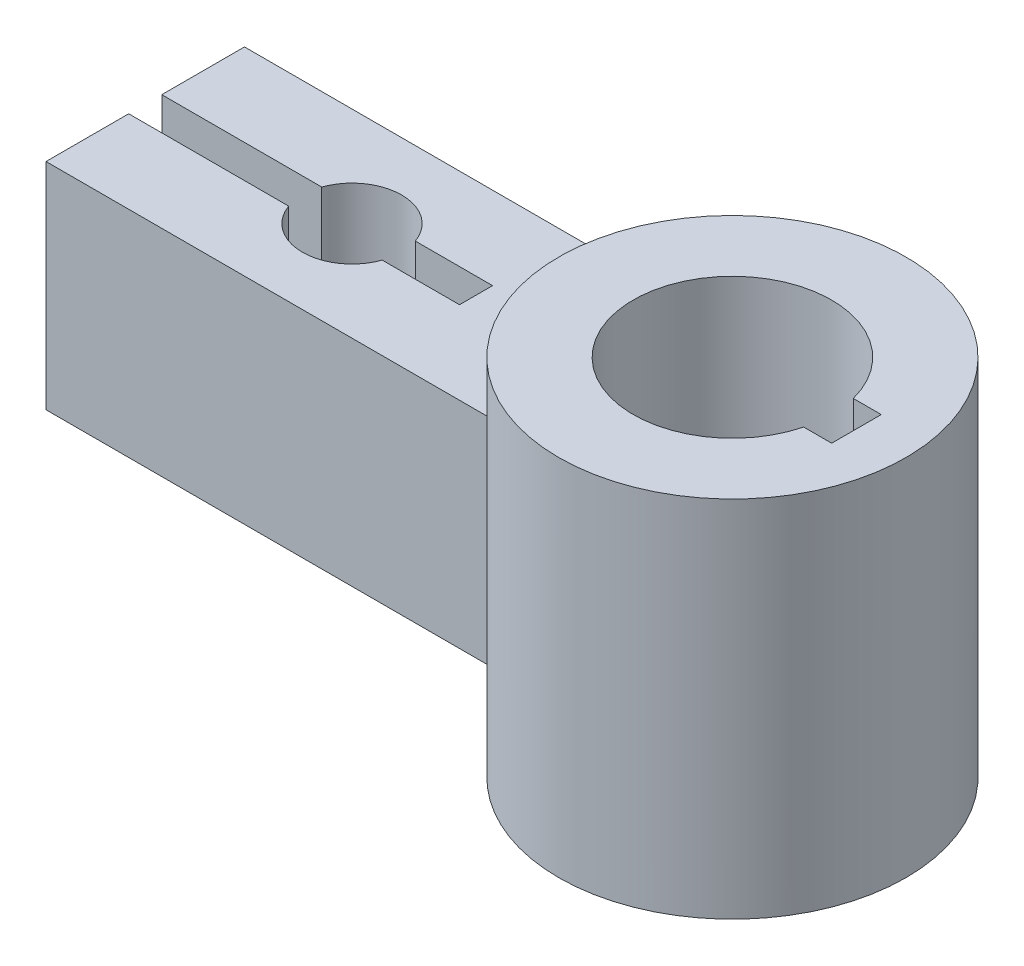
ISO-10303-21;
HEADER;
FILE_DESCRIPTION(('STEP AP214'),'2;1');
FILE_NAME('part.step','',(''),(''),'','','');
FILE_SCHEMA(('AUTOMOTIVE_DESIGN { 1 0 10303 214 1 1 1 1 }'));
ENDSEC;
DATA;
#1=APPLICATION_CONTEXT('core data for automotive mechanical design processes');
#2=APPLICATION_PROTOCOL_DEFINITION('international standard','automotive_design',2000,#1);
#3=PRODUCT_CONTEXT('',#1,'mechanical');
#4=PRODUCT('Part','Part','',(#3));
#5=PRODUCT_RELATED_PRODUCT_CATEGORY('part','',(#4));
#6=PRODUCT_DEFINITION_FORMATION('','',#4);
#7=PRODUCT_DEFINITION_CONTEXT('part definition',#1,'design');
#8=PRODUCT_DEFINITION('design','',#6,#7);
#9=PRODUCT_DEFINITION_SHAPE('','',#8);
#10=(LENGTH_UNIT() NAMED_UNIT(*) SI_UNIT(.MILLI.,.METRE.));
#11=(NAMED_UNIT(*) PLANE_ANGLE_UNIT() SI_UNIT($,.RADIAN.));
#12=(NAMED_UNIT(*) SI_UNIT($,.STERADIAN.) SOLID_ANGLE_UNIT());
#13=UNCERTAINTY_MEASURE_WITH_UNIT(LENGTH_MEASURE(1.E-05),#10,'distance_accuracy_value','');
#14=(GEOMETRIC_REPRESENTATION_CONTEXT(3) GLOBAL_UNCERTAINTY_ASSIGNED_CONTEXT((#13)) GLOBAL_UNIT_ASSIGNED_CONTEXT((#10,
#11,#12)) REPRESENTATION_CONTEXT('',''));
#15=CARTESIAN_POINT('',(0.,0.,0.));
#16=DIRECTION('',(0.,0.,1.));
#17=DIRECTION('',(1.,0.,0.));
#18=AXIS2_PLACEMENT_3D('',#15,#16,#17);
#19=CARTESIAN_POINT('',(0.,0.,-24.));
#20=DIRECTION('',(-1.,0.,0.));
#21=DIRECTION('',(0.,0.,1.));
#22=AXIS2_PLACEMENT_3D('',#19,#20,#21);
#23=PLANE('',#22);
#24=DIRECTION('',(0.,1.,0.));
#25=VECTOR('',#24,1.);
#26=CARTESIAN_POINT('',(0.,-4.,-10.));
#27=LINE('',#26,#25);
#28=CARTESIAN_POINT('',(0.,0.,-10.));
#29=VERTEX_POINT('',#28);
#30=CARTESIAN_POINT('',(0.,26.,-10.));
#31=VERTEX_POINT('',#30);
#32=EDGE_CURVE('E216',#29,#31,#27,.T.);
#33=ORIENTED_EDGE('',*,*,#32,.F.);
#34=DIRECTION('',(0.,0.,1.));
#35=VECTOR('',#34,1.);
#36=CARTESIAN_POINT('',(0.,0.,-24.));
#37=LINE('',#36,#35);
#38=CARTESIAN_POINT('',(0.,0.,0.));
#39=VERTEX_POINT('',#38);
#40=EDGE_CURVE('E253',#29,#39,#37,.T.);
#41=ORIENTED_EDGE('',*,*,#40,.T.);
#42=DIRECTION('',(0.,-1.,0.));
#43=VECTOR('',#42,1.);
#44=CARTESIAN_POINT('',(0.,0.,0.));
#45=LINE('',#44,#43);
#46=CARTESIAN_POINT('',(0.,26.,0.));
#47=VERTEX_POINT('',#46);
#48=EDGE_CURVE('E236',#47,#39,#45,.T.);
#49=ORIENTED_EDGE('',*,*,#48,.F.);
#50=DIRECTION('',(0.,0.,1.));
#51=VECTOR('',#50,1.);
#52=CARTESIAN_POINT('',(0.,26.,-24.));
#53=LINE('',#52,#51);
#54=EDGE_CURVE('E265',#31,#47,#53,.T.);
#55=ORIENTED_EDGE('',*,*,#54,.F.);
#56=EDGE_LOOP('',(#33,#41,#49,#55));
#57=FACE_BOUND('',#56,.T.);
#58=ADVANCED_FACE('F44',(#57),#23,.T.);
#59=DIRECTION('',(0.,1.,0.));
#60=VECTOR('',#59,1.);
#61=CARTESIAN_POINT('',(0.,-4.,-14.));
#62=LINE('',#61,#60);
#63=CARTESIAN_POINT('',(0.,0.,-14.));
#64=VERTEX_POINT('',#63);
#65=CARTESIAN_POINT('',(0.,26.,-14.));
#66=VERTEX_POINT('',#65);
#67=EDGE_CURVE('E217',#64,#66,#62,.T.);
#68=ORIENTED_EDGE('',*,*,#67,.T.);
#69=CARTESIAN_POINT('',(0.,26.,-24.));
#70=VERTEX_POINT('',#69);
#71=EDGE_CURVE('E256',#70,#66,#53,.T.);
#72=ORIENTED_EDGE('',*,*,#71,.F.);
#73=DIRECTION('',(0.,-1.,0.));
#74=VECTOR('',#73,1.);
#75=CARTESIAN_POINT('',(0.,0.,-24.));
#76=LINE('',#75,#74);
#77=CARTESIAN_POINT('',(0.,0.,-24.));
#78=VERTEX_POINT('',#77);
#79=EDGE_CURVE('E239',#70,#78,#76,.T.);
#80=ORIENTED_EDGE('',*,*,#79,.T.);
#81=EDGE_CURVE('E263',#78,#64,#37,.T.);
#82=ORIENTED_EDGE('',*,*,#81,.T.);
#83=EDGE_LOOP('',(#68,#72,#80,#82));
#84=FACE_BOUND('',#83,.T.);
#85=ADVANCED_FACE('F50',(#84),#23,.T.);
#86=CARTESIAN_POINT('',(0.,26.,-24.));
#87=DIRECTION('',(0.,1.,0.));
#88=DIRECTION('',(0.,0.,1.));
#89=AXIS2_PLACEMENT_3D('',#86,#87,#88);
#90=PLANE('',#89);
#91=DIRECTION('',(1.,0.,0.));
#92=VECTOR('',#91,1.);
#93=CARTESIAN_POINT('',(19.3431457505076,26.,-10.));
#94=LINE('',#93,#92);
#95=CARTESIAN_POINT('',(19.3431457505076,26.,-10.));
#96=VERTEX_POINT('',#95);
#97=EDGE_CURVE('E207',#31,#96,#94,.T.);
#98=ORIENTED_EDGE('',*,*,#97,.F.);
#99=ORIENTED_EDGE('',*,*,#54,.T.);
#100=DIRECTION('',(-1.,0.,0.));
#101=VECTOR('',#100,1.);
#102=CARTESIAN_POINT('',(0.,26.,0.));
#103=LINE('',#102,#101);
#104=CARTESIAN_POINT('',(59.2153903091735,26.,0.));
#105=VERTEX_POINT('',#104);
#106=EDGE_CURVE('E242',#105,#47,#103,.T.);
#107=ORIENTED_EDGE('',*,*,#106,.F.);
#108=CARTESIAN_POINT('',(80.,26.,-3.));
#109=DIRECTION('',(0.,1.,0.));
#110=DIRECTION('',(0.,0.,1.));
#111=AXIS2_PLACEMENT_3D('',#108,#109,#110);
#112=CIRCLE('',#111,21.);
#113=CARTESIAN_POINT('',(80.,26.,-24.));
#114=VERTEX_POINT('',#113);
#115=EDGE_CURVE('E214',#114,#105,#112,.T.);
#116=ORIENTED_EDGE('',*,*,#115,.F.);
#117=DIRECTION('',(-1.,0.,0.));
#118=VECTOR('',#117,1.);
#119=CARTESIAN_POINT('',(0.,26.,-24.));
#120=LINE('',#119,#118);
#121=EDGE_CURVE('E250',#114,#70,#120,.T.);
#122=ORIENTED_EDGE('',*,*,#121,.T.);
#123=ORIENTED_EDGE('',*,*,#71,.T.);
#124=DIRECTION('',(-1.,0.,0.));
#125=VECTOR('',#124,1.);
#126=CARTESIAN_POINT('',(0.,26.,-14.));
#127=LINE('',#126,#125);
#128=CARTESIAN_POINT('',(19.3431457505076,26.,-14.));
#129=VERTEX_POINT('',#128);
#130=EDGE_CURVE('E210',#129,#66,#127,.T.);
#131=ORIENTED_EDGE('',*,*,#130,.F.);
#132=CARTESIAN_POINT('',(25.,26.,-12.));
#133=DIRECTION('',(0.,1.,0.));
#134=DIRECTION('',(0.,0.,1.));
#135=AXIS2_PLACEMENT_3D('',#132,#133,#134);
#136=CIRCLE('',#135,6.);
#137=CARTESIAN_POINT('',(30.6568542494924,26.,-14.));
#138=VERTEX_POINT('',#137);
#139=EDGE_CURVE('E204',#138,#129,#136,.T.);
#140=ORIENTED_EDGE('',*,*,#139,.F.);
#141=DIRECTION('',(-1.,0.,0.));
#142=VECTOR('',#141,1.);
#143=CARTESIAN_POINT('',(30.6568542494924,26.,-14.));
#144=LINE('',#143,#142);
#145=CARTESIAN_POINT('',(40.,26.,-14.));
#146=VERTEX_POINT('',#145);
#147=EDGE_CURVE('E203',#146,#138,#144,.T.);
#148=ORIENTED_EDGE('',*,*,#147,.F.);
#149=DIRECTION('',(0.,0.,-1.));
#150=VECTOR('',#149,1.);
#151=CARTESIAN_POINT('',(40.,26.,-14.));
#152=LINE('',#151,#150);
#153=CARTESIAN_POINT('',(40.,26.,-10.));
#154=VERTEX_POINT('',#153);
#155=EDGE_CURVE('E196',#154,#146,#152,.T.);
#156=ORIENTED_EDGE('',*,*,#155,.F.);
#157=DIRECTION('',(1.,0.,0.));
#158=VECTOR('',#157,1.);
#159=CARTESIAN_POINT('',(40.,26.,-10.));
#160=LINE('',#159,#158);
#161=CARTESIAN_POINT('',(30.6568542494924,26.,-10.));
#162=VERTEX_POINT('',#161);
#163=EDGE_CURVE('E192',#162,#154,#160,.T.);
#164=ORIENTED_EDGE('',*,*,#163,.F.);
#165=CARTESIAN_POINT('',(25.,26.,-12.));
#166=DIRECTION('',(0.,1.,0.));
#167=DIRECTION('',(0.,0.,1.));
#168=AXIS2_PLACEMENT_3D('',#165,#166,#167);
#169=CIRCLE('',#168,6.);
#170=EDGE_CURVE('E191',#96,#162,#169,.T.);
#171=ORIENTED_EDGE('',*,*,#170,.F.);
#172=EDGE_LOOP('',(#98,#99,#107,#116,#122,#123,#131,#140,#148,#156,#164,#171));
#173=FACE_BOUND('',#172,.T.);
#174=ADVANCED_FACE('F298',(#173),#90,.T.);
#175=CARTESIAN_POINT('',(0.,0.,-24.));
#176=DIRECTION('',(0.,-1.,0.));
#177=DIRECTION('',(0.,0.,-1.));
#178=AXIS2_PLACEMENT_3D('',#175,#176,#177);
#179=PLANE('',#178);
#180=CARTESIAN_POINT('',(80.,0.,-3.));
#181=DIRECTION('',(0.,-1.,0.));
#182=DIRECTION('',(0.,0.,-1.));
#183=AXIS2_PLACEMENT_3D('',#180,#181,#182);
#184=CIRCLE('',#183,12.);
#185=CARTESIAN_POINT('',(91.6189500386222,0.,0.));
#186=VERTEX_POINT('',#185);
#187=CARTESIAN_POINT('',(91.6189500386222,0.,-6.));
#188=VERTEX_POINT('',#187);
#189=EDGE_CURVE('E189',#186,#188,#184,.T.);
#190=ORIENTED_EDGE('',*,*,#189,.F.);
#191=DIRECTION('',(-1.,0.,0.));
#192=VECTOR('',#191,1.);
#193=CARTESIAN_POINT('',(0.,0.,0.));
#194=LINE('',#193,#192);
#195=CARTESIAN_POINT('',(95.,0.,0.));
#196=VERTEX_POINT('',#195);
#197=EDGE_CURVE('E181',#196,#186,#194,.T.);
#198=ORIENTED_EDGE('',*,*,#197,.F.);
#199=DIRECTION('',(0.,0.,1.));
#200=VECTOR('',#199,1.);
#201=CARTESIAN_POINT('',(95.,0.,-24.));
#202=LINE('',#201,#200);
#203=CARTESIAN_POINT('',(95.,0.,-6.));
#204=VERTEX_POINT('',#203);
#205=EDGE_CURVE('E162',#204,#196,#202,.T.);
#206=ORIENTED_EDGE('',*,*,#205,.F.);
#207=DIRECTION('',(1.,0.,0.));
#208=VECTOR('',#207,1.);
#209=CARTESIAN_POINT('',(0.,0.,-6.));
#210=LINE('',#209,#208);
#211=EDGE_CURVE('E187',#188,#204,#210,.T.);
#212=ORIENTED_EDGE('',*,*,#211,.F.);
#213=EDGE_LOOP('',(#190,#198,#206,#212));
#214=FACE_BOUND('',#213,.T.);
#215=DIRECTION('',(-1.,0.,0.));
#216=VECTOR('',#215,1.);
#217=CARTESIAN_POINT('',(0.,0.,-10.));
#218=LINE('',#217,#216);
#219=CARTESIAN_POINT('',(19.3431457505076,0.,-10.));
#220=VERTEX_POINT('',#219);
#221=EDGE_CURVE('E11',#220,#29,#218,.T.);
#222=ORIENTED_EDGE('',*,*,#221,.F.);
#223=CARTESIAN_POINT('',(25.,0.,-12.));
#224=DIRECTION('',(0.,-1.,0.));
#225=DIRECTION('',(0.,0.,-1.));
#226=AXIS2_PLACEMENT_3D('',#223,#224,#225);
#227=CIRCLE('',#226,6.);
#228=CARTESIAN_POINT('',(30.6568542494924,0.,-10.));
#229=VERTEX_POINT('',#228);
#230=EDGE_CURVE('E52',#229,#220,#227,.T.);
#231=ORIENTED_EDGE('',*,*,#230,.F.);
#232=DIRECTION('',(-1.,0.,0.));
#233=VECTOR('',#232,1.);
#234=CARTESIAN_POINT('',(0.,0.,-10.));
#235=LINE('',#234,#233);
#236=CARTESIAN_POINT('',(40.,0.,-10.));
#237=VERTEX_POINT('',#236);
#238=EDGE_CURVE('E268',#237,#229,#235,.T.);
#239=ORIENTED_EDGE('',*,*,#238,.F.);
#240=DIRECTION('',(0.,0.,1.));
#241=VECTOR('',#240,1.);
#242=CARTESIAN_POINT('',(40.,0.,-24.));
#243=LINE('',#242,#241);
#244=CARTESIAN_POINT('',(40.,0.,-14.));
#245=VERTEX_POINT('',#244);
#246=EDGE_CURVE('E269',#245,#237,#243,.T.);
#247=ORIENTED_EDGE('',*,*,#246,.F.);
#248=DIRECTION('',(1.,0.,0.));
#249=VECTOR('',#248,1.);
#250=CARTESIAN_POINT('',(0.,0.,-14.));
#251=LINE('',#250,#249);
#252=CARTESIAN_POINT('',(30.6568542494924,0.,-14.));
#253=VERTEX_POINT('',#252);
#254=EDGE_CURVE('E272',#253,#245,#251,.T.);
#255=ORIENTED_EDGE('',*,*,#254,.F.);
#256=CARTESIAN_POINT('',(25.,0.,-12.));
#257=DIRECTION('',(0.,-1.,0.));
#258=DIRECTION('',(0.,0.,-1.));
#259=AXIS2_PLACEMENT_3D('',#256,#257,#258);
#260=CIRCLE('',#259,6.);
#261=CARTESIAN_POINT('',(19.3431457505076,0.,-14.));
#262=VERTEX_POINT('',#261);
#263=EDGE_CURVE('E274',#262,#253,#260,.T.);
#264=ORIENTED_EDGE('',*,*,#263,.F.);
#265=DIRECTION('',(1.,0.,0.));
#266=VECTOR('',#265,1.);
#267=CARTESIAN_POINT('',(0.,0.,-14.));
#268=LINE('',#267,#266);
#269=EDGE_CURVE('E280',#64,#262,#268,.T.);
#270=ORIENTED_EDGE('',*,*,#269,.F.);
#271=ORIENTED_EDGE('',*,*,#81,.F.);
#272=DIRECTION('',(1.,0.,0.));
#273=VECTOR('',#272,1.);
#274=CARTESIAN_POINT('',(0.,0.,-24.));
#275=LINE('',#274,#273);
#276=CARTESIAN_POINT('',(80.,0.,-24.));
#277=VERTEX_POINT('',#276);
#278=EDGE_CURVE('E245',#78,#277,#275,.T.);
#279=ORIENTED_EDGE('',*,*,#278,.T.);
#280=CARTESIAN_POINT('',(80.,0.,-3.));
#281=DIRECTION('',(0.,1.,0.));
#282=DIRECTION('',(0.,0.,1.));
#283=AXIS2_PLACEMENT_3D('',#280,#281,#282);
#284=CIRCLE('',#283,21.);
#285=CARTESIAN_POINT('',(59.2153903091735,0.,0.));
#286=VERTEX_POINT('',#285);
#287=EDGE_CURVE('E235',#286,#277,#284,.T.);
#288=ORIENTED_EDGE('',*,*,#287,.F.);
#289=DIRECTION('',(1.,0.,0.));
#290=VECTOR('',#289,1.);
#291=CARTESIAN_POINT('',(0.,0.,0.));
#292=LINE('',#291,#290);
#293=EDGE_CURVE('E255',#39,#286,#292,.T.);
#294=ORIENTED_EDGE('',*,*,#293,.F.);
#295=ORIENTED_EDGE('',*,*,#40,.F.);
#296=EDGE_LOOP('',(#222,#231,#239,#247,#255,#264,#270,#271,#279,#288,#294,#295));
#297=FACE_BOUND('',#296,.T.);
#298=ADVANCED_FACE('F295',(#214,#297),#179,.T.);
#299=CARTESIAN_POINT('',(0.,0.,-24.));
#300=DIRECTION('',(0.,0.,-1.));
#301=DIRECTION('',(-1.,0.,0.));
#302=AXIS2_PLACEMENT_3D('',#299,#300,#301);
#303=PLANE('',#302);
#304=ORIENTED_EDGE('',*,*,#79,.F.);
#305=ORIENTED_EDGE('',*,*,#121,.F.);
#306=DIRECTION('',(0.,1.,0.));
#307=VECTOR('',#306,1.);
#308=CARTESIAN_POINT('',(80.,26.,-24.));
#309=LINE('',#308,#307);
#310=EDGE_CURVE('E249',#277,#114,#309,.T.);
#311=ORIENTED_EDGE('',*,*,#310,.F.);
#312=ORIENTED_EDGE('',*,*,#278,.F.);
#313=EDGE_LOOP('',(#304,#305,#311,#312));
#314=FACE_BOUND('',#313,.T.);
#315=ADVANCED_FACE('F326',(#314),#303,.T.);
#316=CARTESIAN_POINT('',(0.,0.,0.));
#317=DIRECTION('',(0.,0.,-1.));
#318=DIRECTION('',(-1.,0.,0.));
#319=AXIS2_PLACEMENT_3D('',#316,#317,#318);
#320=PLANE('',#319);
#321=ORIENTED_EDGE('',*,*,#293,.T.);
#322=DIRECTION('',(0.,1.,0.));
#323=VECTOR('',#322,1.);
#324=CARTESIAN_POINT('',(59.2153903091735,0.,0.));
#325=LINE('',#324,#323);
#326=EDGE_CURVE('E261',#286,#105,#325,.T.);
#327=ORIENTED_EDGE('',*,*,#326,.T.);
#328=ORIENTED_EDGE('',*,*,#106,.T.);
#329=ORIENTED_EDGE('',*,*,#48,.T.);
#330=EDGE_LOOP('',(#321,#327,#328,#329));
#331=FACE_BOUND('',#330,.T.);
#332=ADVANCED_FACE('F334',(#331),#320,.F.);
#333=CARTESIAN_POINT('',(80.,0.,-3.));
#334=DIRECTION('',(0.,1.,0.));
#335=DIRECTION('',(0.,0.,1.));
#336=AXIS2_PLACEMENT_3D('',#333,#334,#335);
#337=CYLINDRICAL_SURFACE('',#336,21.);
#338=ORIENTED_EDGE('',*,*,#287,.T.);
#339=ORIENTED_EDGE('',*,*,#310,.T.);
#340=ORIENTED_EDGE('',*,*,#115,.T.);
#341=ORIENTED_EDGE('',*,*,#326,.F.);
#342=EDGE_LOOP('',(#338,#339,#340,#341));
#343=FACE_BOUND('',#342,.T.);
#344=CARTESIAN_POINT('',(80.,44.,-3.));
#345=DIRECTION('',(0.,1.,0.));
#346=DIRECTION('',(0.,0.,1.));
#347=AXIS2_PLACEMENT_3D('',#344,#345,#346);
#348=CIRCLE('',#347,21.);
#349=CARTESIAN_POINT('',(80.,44.,18.));
#350=VERTEX_POINT('',#349);
#351=EDGE_CURVE('E229',#350,#350,#348,.T.);
#352=ORIENTED_EDGE('',*,*,#351,.F.);
#353=EDGE_LOOP('',(#352));
#354=FACE_BOUND('',#353,.T.);
#355=ADVANCED_FACE('F329',(#343,#354),#337,.T.);
#356=CARTESIAN_POINT('',(80.,44.,-3.));
#357=DIRECTION('',(0.,1.,0.));
#358=DIRECTION('',(0.,0.,1.));
#359=AXIS2_PLACEMENT_3D('',#356,#357,#358);
#360=PLANE('',#359);
#361=CARTESIAN_POINT('',(80.,44.,-3.));
#362=DIRECTION('',(0.,1.,0.));
#363=DIRECTION('',(0.,0.,1.));
#364=AXIS2_PLACEMENT_3D('',#361,#362,#363);
#365=CIRCLE('',#364,12.);
#366=CARTESIAN_POINT('',(91.6189500386222,44.,-6.));
#367=VERTEX_POINT('',#366);
#368=CARTESIAN_POINT('',(91.6189500386222,44.,0.));
#369=VERTEX_POINT('',#368);
#370=EDGE_CURVE('E70',#367,#369,#365,.T.);
#371=ORIENTED_EDGE('',*,*,#370,.F.);
#372=DIRECTION('',(-1.,0.,0.));
#373=VECTOR('',#372,1.);
#374=CARTESIAN_POINT('',(95.,44.,-6.));
#375=LINE('',#374,#373);
#376=CARTESIAN_POINT('',(95.,44.,-6.));
#377=VERTEX_POINT('',#376);
#378=EDGE_CURVE('E179',#377,#367,#375,.T.);
#379=ORIENTED_EDGE('',*,*,#378,.F.);
#380=DIRECTION('',(0.,0.,-1.));
#381=VECTOR('',#380,1.);
#382=CARTESIAN_POINT('',(95.,44.,-6.));
#383=LINE('',#382,#381);
#384=CARTESIAN_POINT('',(95.,44.,0.));
#385=VERTEX_POINT('',#384);
#386=EDGE_CURVE('E159',#385,#377,#383,.T.);
#387=ORIENTED_EDGE('',*,*,#386,.F.);
#388=DIRECTION('',(1.,0.,0.));
#389=VECTOR('',#388,1.);
#390=CARTESIAN_POINT('',(91.6189500386222,44.,0.));
#391=LINE('',#390,#389);
#392=EDGE_CURVE('E166',#369,#385,#391,.T.);
#393=ORIENTED_EDGE('',*,*,#392,.F.);
#394=EDGE_LOOP('',(#371,#379,#387,#393));
#395=FACE_BOUND('',#394,.T.);
#396=ORIENTED_EDGE('',*,*,#351,.T.);
#397=EDGE_LOOP('',(#396));
#398=FACE_BOUND('',#397,.T.);
#399=ADVANCED_FACE('F172',(#395,#398),#360,.T.);
#400=CARTESIAN_POINT('',(25.,-4.,-12.));
#401=DIRECTION('',(0.,1.,0.));
#402=DIRECTION('',(0.,0.,1.));
#403=AXIS2_PLACEMENT_3D('',#400,#401,#402);
#404=CYLINDRICAL_SURFACE('',#403,6.);
#405=ORIENTED_EDGE('',*,*,#230,.T.);
#406=DIRECTION('',(0.,1.,0.));
#407=VECTOR('',#406,1.);
#408=CARTESIAN_POINT('',(19.3431457505076,-4.,-10.));
#409=LINE('',#408,#407);
#410=EDGE_CURVE('E213',#220,#96,#409,.T.);
#411=ORIENTED_EDGE('',*,*,#410,.T.);
#412=ORIENTED_EDGE('',*,*,#170,.T.);
#413=DIRECTION('',(0.,1.,0.));
#414=VECTOR('',#413,1.);
#415=CARTESIAN_POINT('',(30.6568542494924,-4.,-10.));
#416=LINE('',#415,#414);
#417=EDGE_CURVE('E215',#229,#162,#416,.T.);
#418=ORIENTED_EDGE('',*,*,#417,.F.);
#419=EDGE_LOOP('',(#405,#411,#412,#418));
#420=FACE_BOUND('',#419,.T.);
#421=ADVANCED_FACE('F285',(#420),#404,.F.);
#422=CARTESIAN_POINT('',(19.3431457505076,-4.,-10.));
#423=DIRECTION('',(0.,0.,1.));
#424=DIRECTION('',(1.,0.,0.));
#425=AXIS2_PLACEMENT_3D('',#422,#423,#424);
#426=PLANE('',#425);
#427=ORIENTED_EDGE('',*,*,#221,.T.);
#428=ORIENTED_EDGE('',*,*,#32,.T.);
#429=ORIENTED_EDGE('',*,*,#97,.T.);
#430=ORIENTED_EDGE('',*,*,#410,.F.);
#431=EDGE_LOOP('',(#427,#428,#429,#430));
#432=FACE_BOUND('',#431,.T.);
#433=ADVANCED_FACE('F286',(#432),#426,.F.);
#434=CARTESIAN_POINT('',(0.,-4.,-14.));
#435=DIRECTION('',(0.,0.,-1.));
#436=DIRECTION('',(-1.,0.,0.));
#437=AXIS2_PLACEMENT_3D('',#434,#435,#436);
#438=PLANE('',#437);
#439=ORIENTED_EDGE('',*,*,#269,.T.);
#440=DIRECTION('',(0.,1.,0.));
#441=VECTOR('',#440,1.);
#442=CARTESIAN_POINT('',(19.3431457505076,-4.,-14.));
#443=LINE('',#442,#441);
#444=EDGE_CURVE('E222',#262,#129,#443,.T.);
#445=ORIENTED_EDGE('',*,*,#444,.T.);
#446=ORIENTED_EDGE('',*,*,#130,.T.);
#447=ORIENTED_EDGE('',*,*,#67,.F.);
#448=EDGE_LOOP('',(#439,#445,#446,#447));
#449=FACE_BOUND('',#448,.T.);
#450=ADVANCED_FACE('F376',(#449),#438,.F.);
#451=CARTESIAN_POINT('',(25.,-4.,-12.));
#452=DIRECTION('',(0.,1.,0.));
#453=DIRECTION('',(0.,0.,1.));
#454=AXIS2_PLACEMENT_3D('',#451,#452,#453);
#455=CYLINDRICAL_SURFACE('',#454,6.);
#456=ORIENTED_EDGE('',*,*,#263,.T.);
#457=DIRECTION('',(0.,1.,0.));
#458=VECTOR('',#457,1.);
#459=CARTESIAN_POINT('',(30.6568542494924,-4.,-14.));
#460=LINE('',#459,#458);
#461=EDGE_CURVE('E224',#253,#138,#460,.T.);
#462=ORIENTED_EDGE('',*,*,#461,.T.);
#463=ORIENTED_EDGE('',*,*,#139,.T.);
#464=ORIENTED_EDGE('',*,*,#444,.F.);
#465=EDGE_LOOP('',(#456,#462,#463,#464));
#466=FACE_BOUND('',#465,.T.);
#467=ADVANCED_FACE('F316',(#466),#455,.F.);
#468=CARTESIAN_POINT('',(30.6568542494924,-4.,-14.));
#469=DIRECTION('',(0.,0.,-1.));
#470=DIRECTION('',(-1.,0.,0.));
#471=AXIS2_PLACEMENT_3D('',#468,#469,#470);
#472=PLANE('',#471);
#473=ORIENTED_EDGE('',*,*,#254,.T.);
#474=DIRECTION('',(0.,1.,0.));
#475=VECTOR('',#474,1.);
#476=CARTESIAN_POINT('',(40.,-4.,-14.));
#477=LINE('',#476,#475);
#478=EDGE_CURVE('E223',#245,#146,#477,.T.);
#479=ORIENTED_EDGE('',*,*,#478,.T.);
#480=ORIENTED_EDGE('',*,*,#147,.T.);
#481=ORIENTED_EDGE('',*,*,#461,.F.);
#482=EDGE_LOOP('',(#473,#479,#480,#481));
#483=FACE_BOUND('',#482,.T.);
#484=ADVANCED_FACE('F315',(#483),#472,.F.);
#485=CARTESIAN_POINT('',(40.,-4.,-14.));
#486=DIRECTION('',(1.,0.,0.));
#487=DIRECTION('',(0.,0.,-1.));
#488=AXIS2_PLACEMENT_3D('',#485,#486,#487);
#489=PLANE('',#488);
#490=ORIENTED_EDGE('',*,*,#246,.T.);
#491=DIRECTION('',(0.,1.,0.));
#492=VECTOR('',#491,1.);
#493=CARTESIAN_POINT('',(40.,-4.,-10.));
#494=LINE('',#493,#492);
#495=EDGE_CURVE('E230',#237,#154,#494,.T.);
#496=ORIENTED_EDGE('',*,*,#495,.T.);
#497=ORIENTED_EDGE('',*,*,#155,.T.);
#498=ORIENTED_EDGE('',*,*,#478,.F.);
#499=EDGE_LOOP('',(#490,#496,#497,#498));
#500=FACE_BOUND('',#499,.T.);
#501=ADVANCED_FACE('F309',(#500),#489,.F.);
#502=CARTESIAN_POINT('',(40.,-4.,-10.));
#503=DIRECTION('',(0.,0.,1.));
#504=DIRECTION('',(1.,0.,0.));
#505=AXIS2_PLACEMENT_3D('',#502,#503,#504);
#506=PLANE('',#505);
#507=ORIENTED_EDGE('',*,*,#238,.T.);
#508=ORIENTED_EDGE('',*,*,#417,.T.);
#509=ORIENTED_EDGE('',*,*,#163,.T.);
#510=ORIENTED_EDGE('',*,*,#495,.F.);
#511=EDGE_LOOP('',(#507,#508,#509,#510));
#512=FACE_BOUND('',#511,.T.);
#513=ADVANCED_FACE('F303',(#512),#506,.F.);
#514=CARTESIAN_POINT('',(80.,-6.00000000000001,-3.));
#515=DIRECTION('',(0.,1.,0.));
#516=DIRECTION('',(0.,0.,1.));
#517=AXIS2_PLACEMENT_3D('',#514,#515,#516);
#518=CYLINDRICAL_SURFACE('',#517,12.);
#519=ORIENTED_EDGE('',*,*,#189,.T.);
#520=DIRECTION('',(0.,1.,0.));
#521=VECTOR('',#520,1.);
#522=CARTESIAN_POINT('',(91.6189500386222,-6.00000000000001,-6.));
#523=LINE('',#522,#521);
#524=EDGE_CURVE('E182',#188,#367,#523,.T.);
#525=ORIENTED_EDGE('',*,*,#524,.T.);
#526=ORIENTED_EDGE('',*,*,#370,.T.);
#527=DIRECTION('',(0.,1.,0.));
#528=VECTOR('',#527,1.);
#529=CARTESIAN_POINT('',(91.6189500386222,-6.00000000000001,0.));
#530=LINE('',#529,#528);
#531=EDGE_CURVE('E167',#186,#369,#530,.T.);
#532=ORIENTED_EDGE('',*,*,#531,.F.);
#533=EDGE_LOOP('',(#519,#525,#526,#532));
#534=FACE_BOUND('',#533,.T.);
#535=ADVANCED_FACE('F357',(#534),#518,.F.);
#536=CARTESIAN_POINT('',(95.,-6.00000000000001,-6.));
#537=DIRECTION('',(0.,0.,-1.));
#538=DIRECTION('',(-1.,0.,0.));
#539=AXIS2_PLACEMENT_3D('',#536,#537,#538);
#540=PLANE('',#539);
#541=ORIENTED_EDGE('',*,*,#211,.T.);
#542=DIRECTION('',(0.,1.,0.));
#543=VECTOR('',#542,1.);
#544=CARTESIAN_POINT('',(95.,-6.00000000000001,-6.));
#545=LINE('',#544,#543);
#546=EDGE_CURVE('E164',#204,#377,#545,.T.);
#547=ORIENTED_EDGE('',*,*,#546,.T.);
#548=ORIENTED_EDGE('',*,*,#378,.T.);
#549=ORIENTED_EDGE('',*,*,#524,.F.);
#550=EDGE_LOOP('',(#541,#547,#548,#549));
#551=FACE_BOUND('',#550,.T.);
#552=ADVANCED_FACE('F362',(#551),#540,.F.);
#553=CARTESIAN_POINT('',(95.,-6.00000000000001,-6.));
#554=DIRECTION('',(1.,0.,0.));
#555=DIRECTION('',(0.,0.,-1.));
#556=AXIS2_PLACEMENT_3D('',#553,#554,#555);
#557=PLANE('',#556);
#558=ORIENTED_EDGE('',*,*,#205,.T.);
#559=DIRECTION('',(0.,1.,0.));
#560=VECTOR('',#559,1.);
#561=CARTESIAN_POINT('',(95.,-6.00000000000001,0.));
#562=LINE('',#561,#560);
#563=EDGE_CURVE('E58',#196,#385,#562,.T.);
#564=ORIENTED_EDGE('',*,*,#563,.T.);
#565=ORIENTED_EDGE('',*,*,#386,.T.);
#566=ORIENTED_EDGE('',*,*,#546,.F.);
#567=EDGE_LOOP('',(#558,#564,#565,#566));
#568=FACE_BOUND('',#567,.T.);
#569=ADVANCED_FACE('F160',(#568),#557,.F.);
#570=CARTESIAN_POINT('',(91.6189500386222,-6.00000000000001,0.));
#571=DIRECTION('',(0.,0.,1.));
#572=DIRECTION('',(1.,0.,0.));
#573=AXIS2_PLACEMENT_3D('',#570,#571,#572);
#574=PLANE('',#573);
#575=ORIENTED_EDGE('',*,*,#197,.T.);
#576=ORIENTED_EDGE('',*,*,#531,.T.);
#577=ORIENTED_EDGE('',*,*,#392,.T.);
#578=ORIENTED_EDGE('',*,*,#563,.F.);
#579=EDGE_LOOP('',(#575,#576,#577,#578));
#580=FACE_BOUND('',#579,.T.);
#581=ADVANCED_FACE('F168',(#580),#574,.F.);
#582=CLOSED_SHELL('',(#58,#85,#174,#298,#315,#332,#355,#399,#421,#433,#450,#467,#484,#501,#513,
#535,#552,#569,#581));
#583=MANIFOLD_SOLID_BREP('B2',#582);
#584=ADVANCED_BREP_SHAPE_REPRESENTATION('',(#18,#583),#14);
#585=SHAPE_DEFINITION_REPRESENTATION(#9,#584);
ENDSEC;
END-ISO-10303-21;
